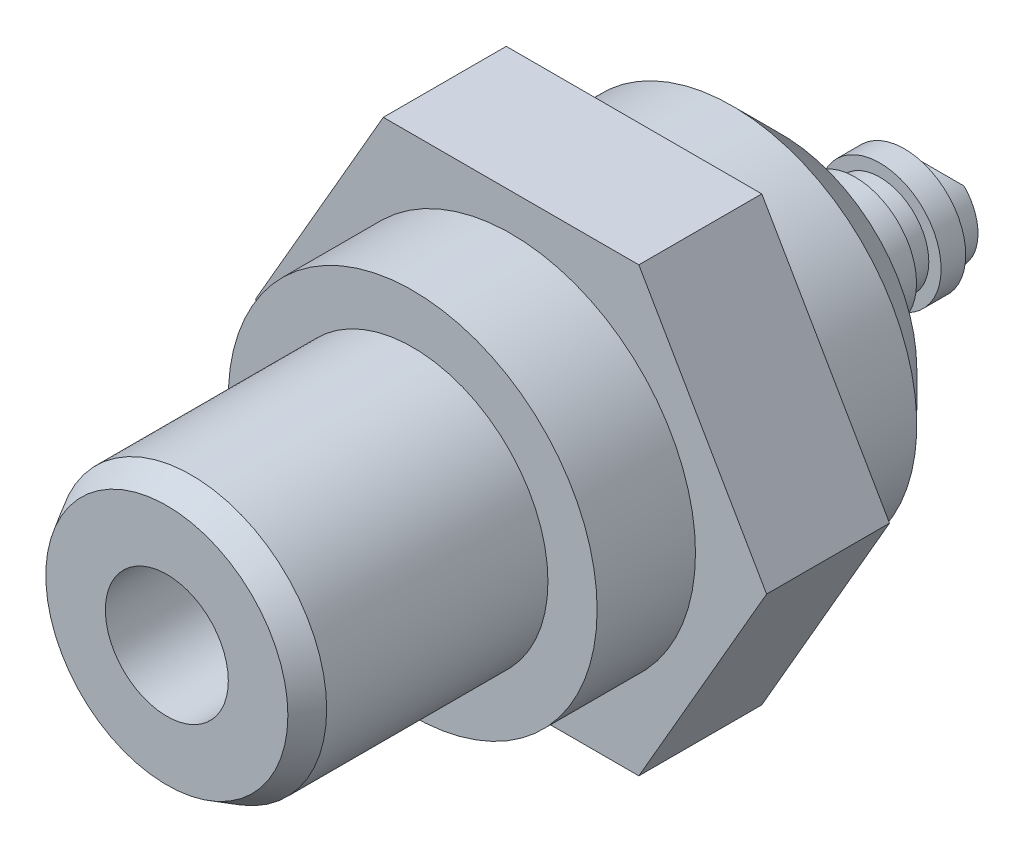
ISO-10303-21;
HEADER;
FILE_DESCRIPTION(('STEP AP214'),'2;1');
FILE_NAME('part.step','',(''),(''),'','','');
FILE_SCHEMA(('AUTOMOTIVE_DESIGN { 1 0 10303 214 1 1 1 1 }'));
ENDSEC;
DATA;
#1=APPLICATION_CONTEXT('core data for automotive mechanical design processes');
#2=APPLICATION_PROTOCOL_DEFINITION('international standard','automotive_design',2000,#1);
#3=PRODUCT_CONTEXT('',#1,'mechanical');
#4=PRODUCT('Part','Part','',(#3));
#5=PRODUCT_RELATED_PRODUCT_CATEGORY('part','',(#4));
#6=PRODUCT_DEFINITION_FORMATION('','',#4);
#7=PRODUCT_DEFINITION_CONTEXT('part definition',#1,'design');
#8=PRODUCT_DEFINITION('design','',#6,#7);
#9=PRODUCT_DEFINITION_SHAPE('','',#8);
#10=(LENGTH_UNIT() NAMED_UNIT(*) SI_UNIT(.MILLI.,.METRE.));
#11=(NAMED_UNIT(*) PLANE_ANGLE_UNIT() SI_UNIT($,.RADIAN.));
#12=(NAMED_UNIT(*) SI_UNIT($,.STERADIAN.) SOLID_ANGLE_UNIT());
#13=UNCERTAINTY_MEASURE_WITH_UNIT(LENGTH_MEASURE(1.E-05),#10,'distance_accuracy_value','');
#14=(GEOMETRIC_REPRESENTATION_CONTEXT(3) GLOBAL_UNCERTAINTY_ASSIGNED_CONTEXT((#13)) GLOBAL_UNIT_ASSIGNED_CONTEXT((#10,
#11,#12)) REPRESENTATION_CONTEXT('',''));
#15=CARTESIAN_POINT('',(0.,0.,0.));
#16=DIRECTION('',(0.,0.,1.));
#17=DIRECTION('',(1.,0.,0.));
#18=AXIS2_PLACEMENT_3D('',#15,#16,#17);
#19=CARTESIAN_POINT('',(5.19615242270663,0.,2.5));
#20=DIRECTION('',(-0.866025403784439,-0.5,0.));
#21=DIRECTION('',(0.5,-0.866025403784439,0.));
#22=AXIS2_PLACEMENT_3D('',#19,#20,#21);
#23=PLANE('',#22);
#24=DIRECTION('',(-0.5,0.866025403784438,0.));
#25=VECTOR('',#24,1.);
#26=CARTESIAN_POINT('',(5.19615242270663,0.,0.));
#27=LINE('',#26,#25);
#28=CARTESIAN_POINT('',(5.19615242270663,0.,0.));
#29=VERTEX_POINT('',#28);
#30=CARTESIAN_POINT('',(2.59807621135332,4.5,0.));
#31=VERTEX_POINT('',#30);
#32=EDGE_CURVE('E138',#29,#31,#27,.T.);
#33=ORIENTED_EDGE('',*,*,#32,.T.);
#34=DIRECTION('',(0.,0.,-1.));
#35=VECTOR('',#34,1.);
#36=CARTESIAN_POINT('',(2.59807621135332,4.5,2.5));
#37=LINE('',#36,#35);
#38=CARTESIAN_POINT('',(2.59807621135332,4.5,2.5));
#39=VERTEX_POINT('',#38);
#40=EDGE_CURVE('E154',#39,#31,#37,.T.);
#41=ORIENTED_EDGE('',*,*,#40,.F.);
#42=DIRECTION('',(-0.5,0.866025403784438,0.));
#43=VECTOR('',#42,1.);
#44=CARTESIAN_POINT('',(5.19615242270663,0.,2.5));
#45=LINE('',#44,#43);
#46=CARTESIAN_POINT('',(5.19615242270663,0.,2.5));
#47=VERTEX_POINT('',#46);
#48=EDGE_CURVE('E146',#47,#39,#45,.T.);
#49=ORIENTED_EDGE('',*,*,#48,.F.);
#50=DIRECTION('',(0.,0.,-1.));
#51=VECTOR('',#50,1.);
#52=CARTESIAN_POINT('',(5.19615242270663,0.,2.5));
#53=LINE('',#52,#51);
#54=EDGE_CURVE('E135',#47,#29,#53,.T.);
#55=ORIENTED_EDGE('',*,*,#54,.T.);
#56=EDGE_LOOP('',(#33,#41,#49,#55));
#57=FACE_BOUND('',#56,.T.);
#58=ADVANCED_FACE('F41',(#57),#23,.F.);
#59=CARTESIAN_POINT('',(2.59807621135332,4.5,2.5));
#60=DIRECTION('',(0.,-1.,0.));
#61=DIRECTION('',(1.,0.,0.));
#62=AXIS2_PLACEMENT_3D('',#59,#60,#61);
#63=PLANE('',#62);
#64=DIRECTION('',(-1.,0.,0.));
#65=VECTOR('',#64,1.);
#66=CARTESIAN_POINT('',(2.59807621135332,4.5,0.));
#67=LINE('',#66,#65);
#68=CARTESIAN_POINT('',(-2.59807621135331,4.5,0.));
#69=VERTEX_POINT('',#68);
#70=EDGE_CURVE('E137',#31,#69,#67,.T.);
#71=ORIENTED_EDGE('',*,*,#70,.T.);
#72=DIRECTION('',(0.,0.,-1.));
#73=VECTOR('',#72,1.);
#74=CARTESIAN_POINT('',(-2.59807621135331,4.5,2.5));
#75=LINE('',#74,#73);
#76=CARTESIAN_POINT('',(-2.59807621135331,4.5,2.5));
#77=VERTEX_POINT('',#76);
#78=EDGE_CURVE('E155',#77,#69,#75,.T.);
#79=ORIENTED_EDGE('',*,*,#78,.F.);
#80=DIRECTION('',(-1.,0.,0.));
#81=VECTOR('',#80,1.);
#82=CARTESIAN_POINT('',(2.59807621135332,4.5,2.5));
#83=LINE('',#82,#81);
#84=EDGE_CURVE('E99',#39,#77,#83,.T.);
#85=ORIENTED_EDGE('',*,*,#84,.F.);
#86=ORIENTED_EDGE('',*,*,#40,.T.);
#87=EDGE_LOOP('',(#71,#79,#85,#86));
#88=FACE_BOUND('',#87,.T.);
#89=ADVANCED_FACE('F195',(#88),#63,.F.);
#90=CARTESIAN_POINT('',(-2.59807621135331,4.5,2.5));
#91=DIRECTION('',(0.866025403784439,-0.5,0.));
#92=DIRECTION('',(0.5,0.866025403784439,0.));
#93=AXIS2_PLACEMENT_3D('',#90,#91,#92);
#94=PLANE('',#93);
#95=DIRECTION('',(-0.5,-0.866025403784439,0.));
#96=VECTOR('',#95,1.);
#97=CARTESIAN_POINT('',(-2.59807621135331,4.5,0.));
#98=LINE('',#97,#96);
#99=CARTESIAN_POINT('',(-5.19615242270663,0.,0.));
#100=VERTEX_POINT('',#99);
#101=EDGE_CURVE('E142',#69,#100,#98,.T.);
#102=ORIENTED_EDGE('',*,*,#101,.T.);
#103=DIRECTION('',(0.,0.,-1.));
#104=VECTOR('',#103,1.);
#105=CARTESIAN_POINT('',(-5.19615242270663,0.,2.5));
#106=LINE('',#105,#104);
#107=CARTESIAN_POINT('',(-5.19615242270663,0.,2.5));
#108=VERTEX_POINT('',#107);
#109=EDGE_CURVE('E130',#108,#100,#106,.T.);
#110=ORIENTED_EDGE('',*,*,#109,.F.);
#111=DIRECTION('',(-0.5,-0.866025403784439,0.));
#112=VECTOR('',#111,1.);
#113=CARTESIAN_POINT('',(-2.59807621135331,4.5,2.5));
#114=LINE('',#113,#112);
#115=EDGE_CURVE('E113',#77,#108,#114,.T.);
#116=ORIENTED_EDGE('',*,*,#115,.F.);
#117=ORIENTED_EDGE('',*,*,#78,.T.);
#118=EDGE_LOOP('',(#102,#110,#116,#117));
#119=FACE_BOUND('',#118,.T.);
#120=ADVANCED_FACE('F196',(#119),#94,.F.);
#121=CARTESIAN_POINT('',(-5.19615242270663,0.,2.5));
#122=DIRECTION('',(0.866025403784439,0.5,0.));
#123=DIRECTION('',(-0.5,0.866025403784439,0.));
#124=AXIS2_PLACEMENT_3D('',#121,#122,#123);
#125=PLANE('',#124);
#126=DIRECTION('',(0.5,-0.866025403784439,0.));
#127=VECTOR('',#126,1.);
#128=CARTESIAN_POINT('',(-5.19615242270663,0.,0.));
#129=LINE('',#128,#127);
#130=CARTESIAN_POINT('',(-2.59807621135331,-4.5,0.));
#131=VERTEX_POINT('',#130);
#132=EDGE_CURVE('E122',#100,#131,#129,.T.);
#133=ORIENTED_EDGE('',*,*,#132,.T.);
#134=DIRECTION('',(0.,0.,-1.));
#135=VECTOR('',#134,1.);
#136=CARTESIAN_POINT('',(-2.59807621135331,-4.5,2.5));
#137=LINE('',#136,#135);
#138=CARTESIAN_POINT('',(-2.59807621135331,-4.5,2.5));
#139=VERTEX_POINT('',#138);
#140=EDGE_CURVE('E123',#139,#131,#137,.T.);
#141=ORIENTED_EDGE('',*,*,#140,.F.);
#142=DIRECTION('',(0.5,-0.866025403784439,0.));
#143=VECTOR('',#142,1.);
#144=CARTESIAN_POINT('',(-5.19615242270663,0.,2.5));
#145=LINE('',#144,#143);
#146=EDGE_CURVE('E107',#108,#139,#145,.T.);
#147=ORIENTED_EDGE('',*,*,#146,.F.);
#148=ORIENTED_EDGE('',*,*,#109,.T.);
#149=EDGE_LOOP('',(#133,#141,#147,#148));
#150=FACE_BOUND('',#149,.T.);
#151=ADVANCED_FACE('F125',(#150),#125,.F.);
#152=CARTESIAN_POINT('',(-2.59807621135331,-4.5,2.5));
#153=DIRECTION('',(0.,1.,0.));
#154=DIRECTION('',(0.,0.,1.));
#155=AXIS2_PLACEMENT_3D('',#152,#153,#154);
#156=PLANE('',#155);
#157=DIRECTION('',(1.,0.,0.));
#158=VECTOR('',#157,1.);
#159=CARTESIAN_POINT('',(-2.59807621135331,-4.5,0.));
#160=LINE('',#159,#158);
#161=CARTESIAN_POINT('',(2.59807621135332,-4.5,0.));
#162=VERTEX_POINT('',#161);
#163=EDGE_CURVE('E144',#131,#162,#160,.T.);
#164=ORIENTED_EDGE('',*,*,#163,.T.);
#165=DIRECTION('',(0.,0.,-1.));
#166=VECTOR('',#165,1.);
#167=CARTESIAN_POINT('',(2.59807621135332,-4.5,2.5));
#168=LINE('',#167,#166);
#169=CARTESIAN_POINT('',(2.59807621135332,-4.5,2.5));
#170=VERTEX_POINT('',#169);
#171=EDGE_CURVE('E126',#170,#162,#168,.T.);
#172=ORIENTED_EDGE('',*,*,#171,.F.);
#173=DIRECTION('',(1.,0.,0.));
#174=VECTOR('',#173,1.);
#175=CARTESIAN_POINT('',(-2.59807621135331,-4.5,2.5));
#176=LINE('',#175,#174);
#177=EDGE_CURVE('E115',#139,#170,#176,.T.);
#178=ORIENTED_EDGE('',*,*,#177,.F.);
#179=ORIENTED_EDGE('',*,*,#140,.T.);
#180=EDGE_LOOP('',(#164,#172,#178,#179));
#181=FACE_BOUND('',#180,.T.);
#182=ADVANCED_FACE('F128',(#181),#156,.F.);
#183=CARTESIAN_POINT('',(2.59807621135332,-4.5,2.5));
#184=DIRECTION('',(-0.866025403784439,0.5,0.));
#185=DIRECTION('',(-0.5,-0.866025403784439,0.));
#186=AXIS2_PLACEMENT_3D('',#183,#184,#185);
#187=PLANE('',#186);
#188=DIRECTION('',(0.5,0.866025403784439,0.));
#189=VECTOR('',#188,1.);
#190=CARTESIAN_POINT('',(2.59807621135332,-4.5,0.));
#191=LINE('',#190,#189);
#192=EDGE_CURVE('E93',#162,#29,#191,.T.);
#193=ORIENTED_EDGE('',*,*,#192,.T.);
#194=ORIENTED_EDGE('',*,*,#54,.F.);
#195=DIRECTION('',(0.5,0.866025403784439,0.));
#196=VECTOR('',#195,1.);
#197=CARTESIAN_POINT('',(2.59807621135332,-4.5,2.5));
#198=LINE('',#197,#196);
#199=EDGE_CURVE('E62',#170,#47,#198,.T.);
#200=ORIENTED_EDGE('',*,*,#199,.F.);
#201=ORIENTED_EDGE('',*,*,#171,.T.);
#202=EDGE_LOOP('',(#193,#194,#200,#201));
#203=FACE_BOUND('',#202,.T.);
#204=ADVANCED_FACE('F246',(#203),#187,.F.);
#205=CARTESIAN_POINT('',(0.,0.,2.5));
#206=DIRECTION('',(0.,0.,1.));
#207=DIRECTION('',(1.,0.,0.));
#208=AXIS2_PLACEMENT_3D('',#205,#206,#207);
#209=PLANE('',#208);
#210=CARTESIAN_POINT('',(0.,0.,2.5));
#211=DIRECTION('',(0.,0.,1.));
#212=DIRECTION('',(1.,0.,0.));
#213=AXIS2_PLACEMENT_3D('',#210,#211,#212);
#214=CIRCLE('',#213,3.75);
#215=CARTESIAN_POINT('',(3.75,0.,2.5));
#216=VERTEX_POINT('',#215);
#217=EDGE_CURVE('E160',#216,#216,#214,.T.);
#218=ORIENTED_EDGE('',*,*,#217,.F.);
#219=EDGE_LOOP('',(#218));
#220=FACE_BOUND('',#219,.T.);
#221=ORIENTED_EDGE('',*,*,#48,.T.);
#222=ORIENTED_EDGE('',*,*,#84,.T.);
#223=ORIENTED_EDGE('',*,*,#115,.T.);
#224=ORIENTED_EDGE('',*,*,#146,.T.);
#225=ORIENTED_EDGE('',*,*,#177,.T.);
#226=ORIENTED_EDGE('',*,*,#199,.T.);
#227=EDGE_LOOP('',(#221,#222,#223,#224,#225,#226));
#228=FACE_BOUND('',#227,.T.);
#229=ADVANCED_FACE('F109',(#220,#228),#209,.T.);
#230=CARTESIAN_POINT('',(0.,0.,0.));
#231=DIRECTION('',(0.,0.,1.));
#232=DIRECTION('',(1.,0.,0.));
#233=AXIS2_PLACEMENT_3D('',#230,#231,#232);
#234=PLANE('',#233);
#235=CARTESIAN_POINT('',(0.,0.,0.));
#236=DIRECTION('',(0.,0.,-1.));
#237=DIRECTION('',(-1.,0.,0.));
#238=AXIS2_PLACEMENT_3D('',#235,#236,#237);
#239=CIRCLE('',#238,3.75);
#240=CARTESIAN_POINT('',(-3.75,0.,0.));
#241=VERTEX_POINT('',#240);
#242=EDGE_CURVE('E164',#241,#241,#239,.T.);
#243=ORIENTED_EDGE('',*,*,#242,.F.);
#244=EDGE_LOOP('',(#243));
#245=FACE_BOUND('',#244,.T.);
#246=ORIENTED_EDGE('',*,*,#32,.F.);
#247=ORIENTED_EDGE('',*,*,#192,.F.);
#248=ORIENTED_EDGE('',*,*,#163,.F.);
#249=ORIENTED_EDGE('',*,*,#132,.F.);
#250=ORIENTED_EDGE('',*,*,#101,.F.);
#251=ORIENTED_EDGE('',*,*,#70,.F.);
#252=EDGE_LOOP('',(#246,#247,#248,#249,#250,#251));
#253=FACE_BOUND('',#252,.T.);
#254=ADVANCED_FACE('F250',(#245,#253),#234,.F.);
#255=CARTESIAN_POINT('',(0.,0.,4.5));
#256=DIRECTION('',(0.,0.,-1.));
#257=DIRECTION('',(-1.,0.,0.));
#258=AXIS2_PLACEMENT_3D('',#255,#256,#257);
#259=CYLINDRICAL_SURFACE('',#258,3.75);
#260=CARTESIAN_POINT('',(0.,0.,4.5));
#261=DIRECTION('',(0.,0.,1.));
#262=DIRECTION('',(1.,0.,0.));
#263=AXIS2_PLACEMENT_3D('',#260,#261,#262);
#264=CIRCLE('',#263,3.75);
#265=CARTESIAN_POINT('',(3.75,0.,4.5));
#266=VERTEX_POINT('',#265);
#267=EDGE_CURVE('E139',#266,#266,#264,.T.);
#268=ORIENTED_EDGE('',*,*,#267,.F.);
#269=EDGE_LOOP('',(#268));
#270=FACE_BOUND('',#269,.T.);
#271=ORIENTED_EDGE('',*,*,#217,.T.);
#272=EDGE_LOOP('',(#271));
#273=FACE_BOUND('',#272,.T.);
#274=ADVANCED_FACE('F300',(#270,#273),#259,.T.);
#275=CARTESIAN_POINT('',(0.,0.,4.5));
#276=DIRECTION('',(0.,0.,1.));
#277=DIRECTION('',(1.,0.,0.));
#278=AXIS2_PLACEMENT_3D('',#275,#276,#277);
#279=PLANE('',#278);
#280=CARTESIAN_POINT('',(0.,0.,4.5));
#281=DIRECTION('',(0.,0.,1.));
#282=DIRECTION('',(1.,0.,0.));
#283=AXIS2_PLACEMENT_3D('',#280,#281,#282);
#284=CIRCLE('',#283,2.75);
#285=CARTESIAN_POINT('',(2.75,0.,4.5));
#286=VERTEX_POINT('',#285);
#287=EDGE_CURVE('E165',#286,#286,#284,.T.);
#288=ORIENTED_EDGE('',*,*,#287,.F.);
#289=EDGE_LOOP('',(#288));
#290=FACE_BOUND('',#289,.T.);
#291=ORIENTED_EDGE('',*,*,#267,.T.);
#292=EDGE_LOOP('',(#291));
#293=FACE_BOUND('',#292,.T.);
#294=ADVANCED_FACE('F223',(#290,#293),#279,.T.);
#295=CARTESIAN_POINT('',(0.,0.,9.5));
#296=DIRECTION('',(0.,0.,-1.));
#297=DIRECTION('',(-1.,0.,0.));
#298=AXIS2_PLACEMENT_3D('',#295,#296,#297);
#299=CYLINDRICAL_SURFACE('',#298,2.75);
#300=CARTESIAN_POINT('',(0.,0.,9.));
#301=DIRECTION('',(0.,0.,1.));
#302=DIRECTION('',(1.,0.,0.));
#303=AXIS2_PLACEMENT_3D('',#300,#301,#302);
#304=CIRCLE('',#303,2.75);
#305=CARTESIAN_POINT('',(2.75,0.,9.));
#306=VERTEX_POINT('',#305);
#307=EDGE_CURVE('E161',#306,#306,#304,.F.);
#308=ORIENTED_EDGE('',*,*,#307,.T.);
#309=EDGE_LOOP('',(#308));
#310=FACE_BOUND('',#309,.T.);
#311=ORIENTED_EDGE('',*,*,#287,.T.);
#312=EDGE_LOOP('',(#311));
#313=FACE_BOUND('',#312,.T.);
#314=ADVANCED_FACE('F216',(#310,#313),#299,.T.);
#315=CARTESIAN_POINT('',(0.,0.,9.5));
#316=DIRECTION('',(0.,0.,1.));
#317=DIRECTION('',(1.,0.,0.));
#318=AXIS2_PLACEMENT_3D('',#315,#316,#317);
#319=PLANE('',#318);
#320=CARTESIAN_POINT('',(0.,0.,9.5));
#321=DIRECTION('',(0.,0.,1.));
#322=DIRECTION('',(1.,0.,0.));
#323=AXIS2_PLACEMENT_3D('',#320,#321,#322);
#324=CIRCLE('',#323,1.25);
#325=CARTESIAN_POINT('',(1.25,0.,9.5));
#326=VERTEX_POINT('',#325);
#327=EDGE_CURVE('E234',#326,#326,#324,.T.);
#328=ORIENTED_EDGE('',*,*,#327,.F.);
#329=EDGE_LOOP('',(#328));
#330=FACE_BOUND('',#329,.T.);
#331=CARTESIAN_POINT('',(0.,0.,9.5));
#332=DIRECTION('',(0.,0.,1.));
#333=DIRECTION('',(1.,0.,0.));
#334=AXIS2_PLACEMENT_3D('',#331,#332,#333);
#335=CIRCLE('',#334,2.46132486540519);
#336=CARTESIAN_POINT('',(2.46132486540519,0.,9.5));
#337=VERTEX_POINT('',#336);
#338=EDGE_CURVE('E158',#337,#337,#335,.T.);
#339=ORIENTED_EDGE('',*,*,#338,.T.);
#340=EDGE_LOOP('',(#339));
#341=FACE_BOUND('',#340,.T.);
#342=ADVANCED_FACE('F210',(#330,#341),#319,.T.);
#343=CARTESIAN_POINT('',(0.,0.,9.5));
#344=DIRECTION('',(0.,0.,-1.));
#345=DIRECTION('',(-1.,0.,0.));
#346=AXIS2_PLACEMENT_3D('',#343,#344,#345);
#347=CONICAL_SURFACE('',#346,2.46132486540519,0.523598775598299);
#348=ORIENTED_EDGE('',*,*,#307,.F.);
#349=EDGE_LOOP('',(#348));
#350=FACE_BOUND('',#349,.T.);
#351=ORIENTED_EDGE('',*,*,#338,.F.);
#352=EDGE_LOOP('',(#351));
#353=FACE_BOUND('',#352,.T.);
#354=ADVANCED_FACE('F205',(#350,#353),#347,.T.);
#355=CARTESIAN_POINT('',(0.,0.,5.5));
#356=DIRECTION('',(0.,0.,1.));
#357=DIRECTION('',(1.,0.,0.));
#358=AXIS2_PLACEMENT_3D('',#355,#356,#357);
#359=CYLINDRICAL_SURFACE('',#358,1.25);
#360=CARTESIAN_POINT('',(0.,0.,5.5));
#361=DIRECTION('',(0.,0.,1.));
#362=DIRECTION('',(1.,0.,0.));
#363=AXIS2_PLACEMENT_3D('',#360,#361,#362);
#364=CIRCLE('',#363,1.25);
#365=CARTESIAN_POINT('',(1.25,0.,5.5));
#366=VERTEX_POINT('',#365);
#367=EDGE_CURVE('E236',#366,#366,#364,.T.);
#368=ORIENTED_EDGE('',*,*,#367,.F.);
#369=EDGE_LOOP('',(#368));
#370=FACE_BOUND('',#369,.T.);
#371=ORIENTED_EDGE('',*,*,#327,.T.);
#372=EDGE_LOOP('',(#371));
#373=FACE_BOUND('',#372,.T.);
#374=ADVANCED_FACE('F206',(#370,#373),#359,.F.);
#375=CARTESIAN_POINT('',(0.,0.,5.5));
#376=DIRECTION('',(0.,0.,1.));
#377=DIRECTION('',(1.,0.,0.));
#378=AXIS2_PLACEMENT_3D('',#375,#376,#377);
#379=PLANE('',#378);
#380=ORIENTED_EDGE('',*,*,#367,.T.);
#381=EDGE_LOOP('',(#380));
#382=FACE_BOUND('',#381,.T.);
#383=ADVANCED_FACE('F190',(#382),#379,.T.);
#384=CARTESIAN_POINT('',(0.,0.,-3.));
#385=DIRECTION('',(0.,0.,1.));
#386=DIRECTION('',(1.,0.,0.));
#387=AXIS2_PLACEMENT_3D('',#384,#385,#386);
#388=CYLINDRICAL_SURFACE('',#387,3.75);
#389=CARTESIAN_POINT('',(0.,0.,-2.));
#390=DIRECTION('',(0.,0.,-1.));
#391=DIRECTION('',(-1.,0.,0.));
#392=AXIS2_PLACEMENT_3D('',#389,#390,#391);
#393=CIRCLE('',#392,3.75);
#394=CARTESIAN_POINT('',(-3.75,0.,-2.));
#395=VERTEX_POINT('',#394);
#396=EDGE_CURVE('E49',#395,#395,#393,.F.);
#397=ORIENTED_EDGE('',*,*,#396,.T.);
#398=EDGE_LOOP('',(#397));
#399=FACE_BOUND('',#398,.T.);
#400=ORIENTED_EDGE('',*,*,#242,.T.);
#401=EDGE_LOOP('',(#400));
#402=FACE_BOUND('',#401,.T.);
#403=ADVANCED_FACE('F173',(#399,#402),#388,.T.);
#404=CARTESIAN_POINT('',(0.,0.,-3.));
#405=DIRECTION('',(0.,0.,-1.));
#406=DIRECTION('',(-1.,0.,0.));
#407=AXIS2_PLACEMENT_3D('',#404,#405,#406);
#408=PLANE('',#407);
#409=CARTESIAN_POINT('',(0.,0.,-3.));
#410=DIRECTION('',(0.,0.,1.));
#411=DIRECTION('',(1.,0.,0.));
#412=AXIS2_PLACEMENT_3D('',#409,#410,#411);
#413=CIRCLE('',#412,1.245);
#414=CARTESIAN_POINT('',(1.245,0.,-3.));
#415=VERTEX_POINT('',#414);
#416=EDGE_CURVE('E475',#415,#415,#413,.T.);
#417=ORIENTED_EDGE('',*,*,#416,.T.);
#418=EDGE_LOOP('',(#417));
#419=FACE_BOUND('',#418,.T.);
#420=CARTESIAN_POINT('',(0.,0.,-3.));
#421=DIRECTION('',(0.,0.,-1.));
#422=DIRECTION('',(-1.,0.,0.));
#423=AXIS2_PLACEMENT_3D('',#420,#421,#422);
#424=CIRCLE('',#423,2.75);
#425=CARTESIAN_POINT('',(-2.75,0.,-3.));
#426=VERTEX_POINT('',#425);
#427=EDGE_CURVE('E167',#426,#426,#424,.T.);
#428=ORIENTED_EDGE('',*,*,#427,.T.);
#429=EDGE_LOOP('',(#428));
#430=FACE_BOUND('',#429,.T.);
#431=ADVANCED_FACE('F180',(#419,#430),#408,.T.);
#432=CARTESIAN_POINT('',(0.,0.,-3.));
#433=DIRECTION('',(0.,0.,1.));
#434=DIRECTION('',(1.,0.,0.));
#435=AXIS2_PLACEMENT_3D('',#432,#433,#434);
#436=CONICAL_SURFACE('',#435,2.75,0.785398163397447);
#437=ORIENTED_EDGE('',*,*,#396,.F.);
#438=EDGE_LOOP('',(#437));
#439=FACE_BOUND('',#438,.T.);
#440=ORIENTED_EDGE('',*,*,#427,.F.);
#441=EDGE_LOOP('',(#440));
#442=FACE_BOUND('',#441,.T.);
#443=ADVANCED_FACE('F42',(#439,#442),#436,.T.);
#444=CARTESIAN_POINT('',(0.,0.,-3.));
#445=DIRECTION('',(0.,0.,1.));
#446=DIRECTION('',(1.,0.,0.));
#447=AXIS2_PLACEMENT_3D('',#444,#445,#446);
#448=CYLINDRICAL_SURFACE('',#447,1.245);
#449=CARTESIAN_POINT('',(0.,0.,-4.5));
#450=DIRECTION('',(0.,0.,1.));
#451=DIRECTION('',(1.,0.,0.));
#452=AXIS2_PLACEMENT_3D('',#449,#450,#451);
#453=CIRCLE('',#452,1.245);
#454=CARTESIAN_POINT('',(1.245,0.,-4.5));
#455=VERTEX_POINT('',#454);
#456=EDGE_CURVE('E473',#455,#455,#453,.T.);
#457=ORIENTED_EDGE('',*,*,#456,.T.);
#458=EDGE_LOOP('',(#457));
#459=FACE_BOUND('',#458,.T.);
#460=ORIENTED_EDGE('',*,*,#416,.F.);
#461=EDGE_LOOP('',(#460));
#462=FACE_BOUND('',#461,.T.);
#463=ADVANCED_FACE('F178',(#459,#462),#448,.T.);
#464=CARTESIAN_POINT('',(0.,-1.245,-4.5));
#465=DIRECTION('',(0.,0.,-1.));
#466=DIRECTION('',(-1.,0.,0.));
#467=AXIS2_PLACEMENT_3D('',#464,#465,#466);
#468=PLANE('',#467);
#469=CARTESIAN_POINT('',(0.,0.,-4.5));
#470=DIRECTION('',(0.,0.,1.));
#471=DIRECTION('',(1.,0.,0.));
#472=AXIS2_PLACEMENT_3D('',#469,#470,#471);
#473=CIRCLE('',#472,0.995);
#474=CARTESIAN_POINT('',(0.995,0.,-4.5));
#475=VERTEX_POINT('',#474);
#476=EDGE_CURVE('E466',#475,#475,#473,.T.);
#477=ORIENTED_EDGE('',*,*,#476,.T.);
#478=EDGE_LOOP('',(#477));
#479=FACE_BOUND('',#478,.T.);
#480=ORIENTED_EDGE('',*,*,#456,.F.);
#481=EDGE_LOOP('',(#480));
#482=FACE_BOUND('',#481,.T.);
#483=ADVANCED_FACE('F366',(#479,#482),#468,.T.);
#484=CARTESIAN_POINT('',(0.,0.,-3.));
#485=DIRECTION('',(0.,0.,1.));
#486=DIRECTION('',(1.,0.,0.));
#487=AXIS2_PLACEMENT_3D('',#484,#485,#486);
#488=CYLINDRICAL_SURFACE('',#487,0.995);
#489=CARTESIAN_POINT('',(0.,0.,-5.));
#490=DIRECTION('',(0.,0.,1.));
#491=DIRECTION('',(1.,0.,0.));
#492=AXIS2_PLACEMENT_3D('',#489,#490,#491);
#493=CIRCLE('',#492,0.995);
#494=CARTESIAN_POINT('',(0.995,0.,-5.));
#495=VERTEX_POINT('',#494);
#496=EDGE_CURVE('E464',#495,#495,#493,.T.);
#497=ORIENTED_EDGE('',*,*,#496,.T.);
#498=EDGE_LOOP('',(#497));
#499=FACE_BOUND('',#498,.T.);
#500=ORIENTED_EDGE('',*,*,#476,.F.);
#501=EDGE_LOOP('',(#500));
#502=FACE_BOUND('',#501,.T.);
#503=ADVANCED_FACE('F380',(#499,#502),#488,.T.);
#504=CARTESIAN_POINT('',(0.,-0.995,-5.));
#505=DIRECTION('',(0.,0.,1.));
#506=DIRECTION('',(1.,0.,0.));
#507=AXIS2_PLACEMENT_3D('',#504,#505,#506);
#508=PLANE('',#507);
#509=CARTESIAN_POINT('',(0.,0.,-5.));
#510=DIRECTION('',(0.,0.,1.));
#511=DIRECTION('',(1.,0.,0.));
#512=AXIS2_PLACEMENT_3D('',#509,#510,#511);
#513=CIRCLE('',#512,1.245);
#514=CARTESIAN_POINT('',(1.245,0.,-5.));
#515=VERTEX_POINT('',#514);
#516=EDGE_CURVE('E465',#515,#515,#513,.T.);
#517=ORIENTED_EDGE('',*,*,#516,.T.);
#518=EDGE_LOOP('',(#517));
#519=FACE_BOUND('',#518,.T.);
#520=ORIENTED_EDGE('',*,*,#496,.F.);
#521=EDGE_LOOP('',(#520));
#522=FACE_BOUND('',#521,.T.);
#523=ADVANCED_FACE('F390',(#519,#522),#508,.T.);
#524=CARTESIAN_POINT('',(0.,0.,-3.));
#525=DIRECTION('',(0.,0.,1.));
#526=DIRECTION('',(1.,0.,0.));
#527=AXIS2_PLACEMENT_3D('',#524,#525,#526);
#528=CYLINDRICAL_SURFACE('',#527,1.245);
#529=CARTESIAN_POINT('',(0.,0.,-5.5));
#530=DIRECTION('',(0.,0.,1.));
#531=DIRECTION('',(1.,0.,0.));
#532=AXIS2_PLACEMENT_3D('',#529,#530,#531);
#533=CIRCLE('',#532,1.245);
#534=CARTESIAN_POINT('',(1.245,0.,-5.5));
#535=VERTEX_POINT('',#534);
#536=EDGE_CURVE('E457',#535,#535,#533,.T.);
#537=ORIENTED_EDGE('',*,*,#536,.T.);
#538=EDGE_LOOP('',(#537));
#539=FACE_BOUND('',#538,.T.);
#540=ORIENTED_EDGE('',*,*,#516,.F.);
#541=EDGE_LOOP('',(#540));
#542=FACE_BOUND('',#541,.T.);
#543=ADVANCED_FACE('F400',(#539,#542),#528,.T.);
#544=CARTESIAN_POINT('',(0.,-1.245,-5.5));
#545=DIRECTION('',(0.,0.,-1.));
#546=DIRECTION('',(-1.,0.,0.));
#547=AXIS2_PLACEMENT_3D('',#544,#545,#546);
#548=PLANE('',#547);
#549=CARTESIAN_POINT('',(0.,0.,-5.5));
#550=DIRECTION('',(0.,0.,1.));
#551=DIRECTION('',(1.,0.,0.));
#552=AXIS2_PLACEMENT_3D('',#549,#550,#551);
#553=CIRCLE('',#552,0.995);
#554=CARTESIAN_POINT('',(0.995,0.,-5.5));
#555=VERTEX_POINT('',#554);
#556=EDGE_CURVE('E451',#555,#555,#553,.T.);
#557=ORIENTED_EDGE('',*,*,#556,.T.);
#558=EDGE_LOOP('',(#557));
#559=FACE_BOUND('',#558,.T.);
#560=ORIENTED_EDGE('',*,*,#536,.F.);
#561=EDGE_LOOP('',(#560));
#562=FACE_BOUND('',#561,.T.);
#563=ADVANCED_FACE('F410',(#559,#562),#548,.T.);
#564=CARTESIAN_POINT('',(0.,0.,-3.));
#565=DIRECTION('',(0.,0.,1.));
#566=DIRECTION('',(1.,0.,0.));
#567=AXIS2_PLACEMENT_3D('',#564,#565,#566);
#568=CYLINDRICAL_SURFACE('',#567,0.995);
#569=CARTESIAN_POINT('',(0.,0.,-6.695));
#570=DIRECTION('',(0.,-0.707106781186547,0.707106781186547));
#571=DIRECTION('',(0.,0.707106781186548,0.707106781186548));
#572=AXIS2_PLACEMENT_3D('',#569,#570,#571);
#573=ELLIPSE('',#572,1.40714249456123,0.995);
#574=CARTESIAN_POINT('',(-0.712039324756717,0.695,-6.));
#575=VERTEX_POINT('',#574);
#576=CARTESIAN_POINT('',(0.712039324756716,0.695,-6.));
#577=VERTEX_POINT('',#576);
#578=EDGE_CURVE('E54',#575,#577,#573,.F.);
#579=ORIENTED_EDGE('',*,*,#578,.F.);
#580=CARTESIAN_POINT('',(0.,0.,-6.));
#581=DIRECTION('',(0.,0.,1.));
#582=DIRECTION('',(1.,0.,0.));
#583=AXIS2_PLACEMENT_3D('',#580,#581,#582);
#584=CIRCLE('',#583,0.995);
#585=EDGE_CURVE('E453',#575,#577,#584,.T.);
#586=ORIENTED_EDGE('',*,*,#585,.T.);
#587=EDGE_LOOP('',(#579,#586));
#588=FACE_BOUND('',#587,.T.);
#589=ORIENTED_EDGE('',*,*,#556,.F.);
#590=EDGE_LOOP('',(#589));
#591=FACE_BOUND('',#590,.T.);
#592=ADVANCED_FACE('F417',(#588,#591),#568,.T.);
#593=CARTESIAN_POINT('',(0.,-0.995,-6.));
#594=DIRECTION('',(0.,0.,-1.));
#595=DIRECTION('',(-1.,0.,0.));
#596=AXIS2_PLACEMENT_3D('',#593,#594,#595);
#597=PLANE('',#596);
#598=DIRECTION('',(-1.,0.,0.));
#599=VECTOR('',#598,1.);
#600=CARTESIAN_POINT('',(0.,0.695,-6.));
#601=LINE('',#600,#599);
#602=EDGE_CURVE('E11',#577,#575,#601,.T.);
#603=ORIENTED_EDGE('',*,*,#602,.F.);
#604=ORIENTED_EDGE('',*,*,#585,.F.);
#605=EDGE_LOOP('',(#603,#604));
#606=FACE_BOUND('',#605,.T.);
#607=ADVANCED_FACE('F430',(#606),#597,.T.);
#608=CARTESIAN_POINT('',(-5.19615242270663,0.695,-6.));
#609=DIRECTION('',(0.,-0.707106781186547,0.707106781186547));
#610=DIRECTION('',(0.,-0.707106781186548,-0.707106781186548));
#611=AXIS2_PLACEMENT_3D('',#608,#609,#610);
#612=PLANE('',#611);
#613=ORIENTED_EDGE('',*,*,#578,.T.);
#614=ORIENTED_EDGE('',*,*,#602,.T.);
#615=EDGE_LOOP('',(#613,#614));
#616=FACE_BOUND('',#615,.T.);
#617=ADVANCED_FACE('F440',(#616),#612,.F.);
#618=CLOSED_SHELL('',(#58,#89,#120,#151,#182,#204,#229,#254,#274,#294,#314,#342,#354,#374,#383,
#403,#431,#443,#463,#483,#503,#523,#543,#563,#592,#607,#617));
#619=MANIFOLD_SOLID_BREP('B2',#618);
#620=ADVANCED_BREP_SHAPE_REPRESENTATION('',(#18,#619),#14);
#621=SHAPE_DEFINITION_REPRESENTATION(#9,#620);
ENDSEC;
END-ISO-10303-21;
